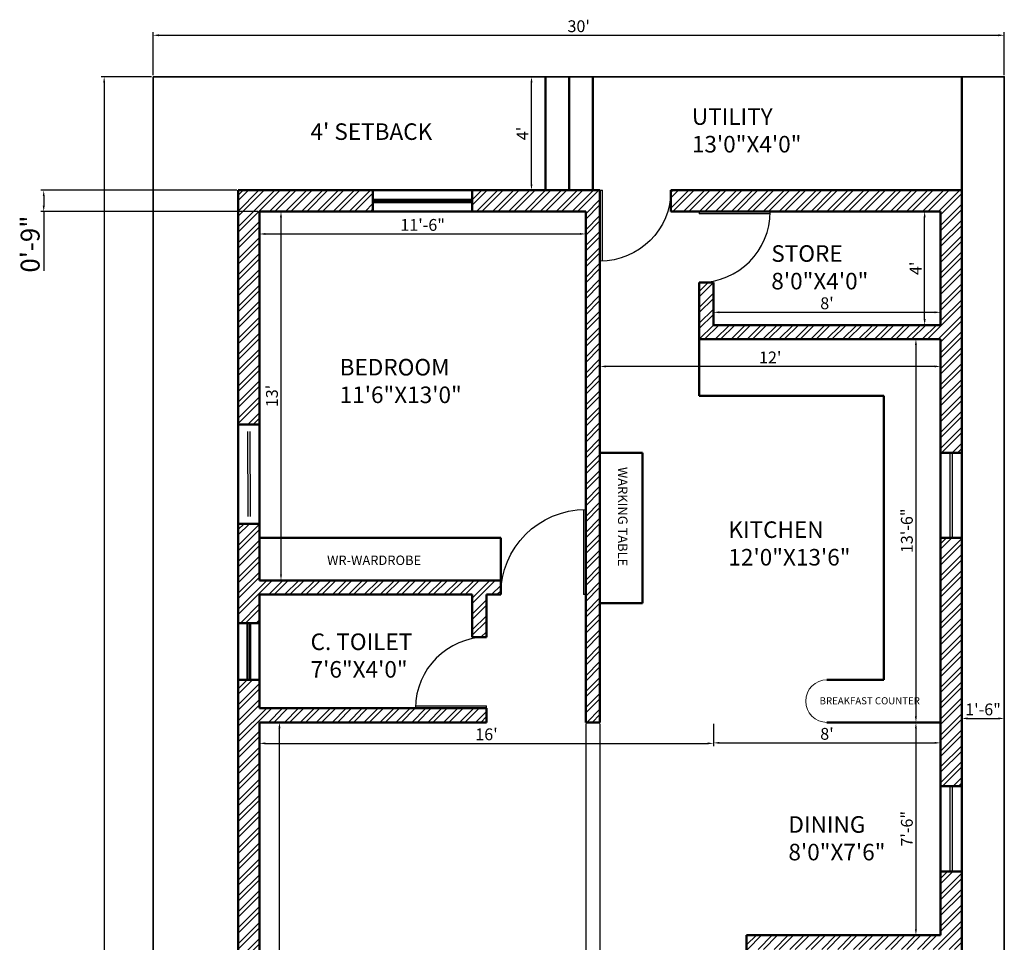
# Model space of a CAD drawing. Units: inches. Extents: x 1986 to 21484, y -1816 to 2016.
# Tile 83 of 85: x 4780 to 5197, y 1535 to 1925. Entities that reach past the tile are written whole.
import ezdxf

# ---------------------------------------------------------------- set-up
doc = ezdxf.new("R2010")
doc.units = ezdxf.units.IN
for name, color, linetype, lineweight in [('A-ANNO-DIMS', 2, 'Continuous', 18), ('A-ANNO-TEXT', 7, 'Continuous', 18), ('A-AREA-IDEN', 3, 'Continuous', 18), ('A-DOOR', 3, 'Continuous', 25), ('A-FURN', 8, 'Continuous', 18), ('A-GLAZ', 4, 'Continuous', 25), ('A-WALL', 7, 'Continuous', 50), ('A-WALL-PATT', 8, 'Continuous', 13), ('C-PROP', 7, 'Continuous', 35)]:
    doc.layers.add(name, color=color, linetype=linetype, lineweight=lineweight)
doc.styles.get("Standard").update_dxf_attribs({"font": 'arial.ttf'})
doc.dimstyles.new('ISO-25', dxfattribs={"dimtxt": 8, "dimasz": 2.5, "dimexe": 1.25, "dimexo": 0.625, "dimtad": 1, "dimdec": 1, "dimlunit": 3, "dimtxsty": 'Standard', "dimcen": 2.5, "dimadec": 0, "dimazin": 0, "dimtfac": 1, "dimtdec": 1, "dimtmove": 0, "dimatfit": 3, "dimfxl": 1, "dimarcsym": 0})

# ---------------------------------------------------------------- blocks, each defined once
blk = doc.blocks.new('D2')
for p, q in [((1722.5, 1505.46), (1722.5, 1475.46)), ((1723.5, 1505.46), (1723.5, 1475.46)), ((1722.5, 1475.46), (1723.5, 1475.46))]:
    blk.add_line(p, q)
blk.add_arc((1722.5, 1475.46), 30, 0, 90)
blk = doc.blocks.new('D1')
for p, q in [((1805.96, 1500.36), (1805.96, 1464.36)), ((1806.96, 1500.36), (1806.96, 1464.36)), ((1805.96, 1464.36), (1806.96, 1464.36))]:
    blk.add_line(p, q)
blk.add_arc((1805.96, 1464.36), 36, 0, 90)
blk = doc.blocks.new('*D35')
at = {"layer": 'A-ANNO-DIMS', "color": 0, "lineweight": -2, "transparency": 16777216}
for p, q in [((4882.51, 1843.75), (4892.24, 1843.75)), ((4890.99, 1690.25), (4890.99, 1841.25)), ((4882.51, 1687.75), (4892.24, 1687.75))]:
    blk.add_line(p, q, dxfattribs=at)
at = {"layer": 'A-ANNO-DIMS', "color": 0, "transparency": 16777216}
for points in [[(4890.57, 1841.25), (4891.4, 1841.25), (4890.99, 1843.75)], [(4890.57, 1690.25), (4891.4, 1690.25), (4890.99, 1687.75)]]:
    blk.add_solid(points, dxfattribs=at)
at = {"layer": 'Defpoints', "color": 0, "transparency": 16777216}
for p in [(4881.89, 1843.75), (4890.99, 1843.75), (4881.89, 1687.75)]:
    blk.add_point(p, dxfattribs=at)
at = {"layer": 'A-ANNO-DIMS', "color": 0, "transparency": 16777216, "insert": (4887.81, 1765.75), "char_height": 5, "attachment_point": 5, "rotation": 90}
blk.add_mtext("13'", dxfattribs=at)
blk = doc.blocks.new('*D36')
at = {"layer": 'A-ANNO-DIMS', "color": 0, "lineweight": -2, "transparency": 16777216}
for p, q in [((4881.89, 1843.13), (4881.89, 1833.02)), ((5019.89, 1843.13), (5019.89, 1833.02)), ((4884.39, 1834.27), (5017.39, 1834.27))]:
    blk.add_line(p, q, dxfattribs=at)
at = {"layer": 'A-ANNO-DIMS', "color": 0, "transparency": 16777216}
for points in [[(4884.39, 1834.68), (4884.39, 1833.85), (4881.89, 1834.27)], [(5017.39, 1834.68), (5017.39, 1833.85), (5019.89, 1834.27)]]:
    blk.add_solid(points, dxfattribs=at)
at = {"layer": 'Defpoints', "color": 0, "transparency": 16777216}
for p in [(4881.89, 1843.75), (5019.89, 1843.75), (5019.89, 1834.27)]:
    blk.add_point(p, dxfattribs=at)
at = {"layer": 'A-ANNO-DIMS', "color": 0, "transparency": 16777216, "insert": (4950.89, 1837.44), "char_height": 5, "attachment_point": 5}
blk.add_mtext('11\'-6"', dxfattribs=at)
blk = doc.blocks.new('*D37')
at = {"layer": 'A-ANNO-DIMS', "color": 0, "lineweight": -2, "transparency": 16777216}
for p, q in [((5169.26, 1843.75), (5161.95, 1843.75)), ((5163.2, 1798.25), (5163.2, 1841.25)), ((5169.26, 1795.75), (5161.95, 1795.75))]:
    blk.add_line(p, q, dxfattribs=at)
at = {"layer": 'A-ANNO-DIMS', "color": 0, "transparency": 16777216}
for points in [[(5162.78, 1841.25), (5163.62, 1841.25), (5163.2, 1843.75)], [(5162.78, 1798.25), (5163.62, 1798.25), (5163.2, 1795.75)]]:
    blk.add_solid(points, dxfattribs=at)
at = {"layer": 'Defpoints', "color": 0, "transparency": 16777216}
for p in [(5163.2, 1843.75), (5169.89, 1843.75), (5169.89, 1795.75)]:
    blk.add_point(p, dxfattribs=at)
at = {"layer": 'A-ANNO-DIMS', "color": 0, "transparency": 16777216, "insert": (5160.07, 1819.75), "char_height": 5, "attachment_point": 5, "rotation": 90}
blk.add_mtext("4'", dxfattribs=at)
blk = doc.blocks.new('*D38')
at = {"layer": 'A-ANNO-DIMS', "color": 0, "lineweight": -2, "transparency": 16777216}
for p, q in [((5073.89, 1796.38), (5073.89, 1802.38)), ((5076.39, 1801.13), (5167.39, 1801.13)), ((5169.89, 1796.38), (5169.89, 1802.38))]:
    blk.add_line(p, q, dxfattribs=at)
at = {"layer": 'A-ANNO-DIMS', "color": 0, "transparency": 16777216}
for points in [[(5076.39, 1801.54), (5076.39, 1800.71), (5073.89, 1801.13)], [(5167.39, 1801.54), (5167.39, 1800.71), (5169.89, 1801.13)]]:
    blk.add_solid(points, dxfattribs=at)
at = {"layer": 'Defpoints', "color": 0, "transparency": 16777216}
for p in [(5169.89, 1801.13), (5073.89, 1795.75), (5169.89, 1795.75)]:
    blk.add_point(p, dxfattribs=at)
at = {"layer": 'A-ANNO-DIMS', "color": 0, "transparency": 16777216, "insert": (5121.89, 1804.31), "char_height": 5, "attachment_point": 5}
blk.add_mtext("8'", dxfattribs=at)
blk = doc.blocks.new('*D39')
at = {"layer": 'A-ANNO-DIMS', "color": 0, "lineweight": -2, "transparency": 16777216}
for p, q in [((5025.89, 1789.13), (5025.89, 1777)), ((5169.89, 1789.13), (5169.89, 1777)), ((5167.39, 1778.25), (5028.39, 1778.25))]:
    blk.add_line(p, q, dxfattribs=at)
at = {"layer": 'A-ANNO-DIMS', "color": 0, "transparency": 16777216}
for points in [[(5028.39, 1778.67), (5028.39, 1777.84), (5025.89, 1778.25)], [(5167.39, 1778.67), (5167.39, 1777.84), (5169.89, 1778.25)]]:
    blk.add_solid(points, dxfattribs=at)
at = {"layer": 'Defpoints', "color": 0, "transparency": 16777216}
for p in [(5025.89, 1789.75), (5169.89, 1789.75), (5025.89, 1778.25)]:
    blk.add_point(p, dxfattribs=at)
at = {"layer": 'A-ANNO-DIMS', "color": 0, "transparency": 16777216, "insert": (5097.89, 1781.39), "char_height": 5, "attachment_point": 5}
blk.add_mtext("12'", dxfattribs=at)
blk = doc.blocks.new('*D40')
at = {"layer": 'A-ANNO-DIMS', "color": 0, "lineweight": -2, "transparency": 16777216}
for p, q in [((5169.26, 1789.75), (5158.26, 1789.75)), ((5159.51, 1787.25), (5159.51, 1630.25)), ((5169.26, 1627.75), (5158.26, 1627.75))]:
    blk.add_line(p, q, dxfattribs=at)
at = {"layer": 'A-ANNO-DIMS', "color": 0, "transparency": 16777216}
for points in [[(5159.09, 1787.25), (5159.92, 1787.25), (5159.51, 1789.75)], [(5159.09, 1630.25), (5159.92, 1630.25), (5159.51, 1627.75)]]:
    blk.add_solid(points, dxfattribs=at)
at = {"layer": 'Defpoints', "color": 0, "transparency": 16777216}
for p in [(5169.89, 1789.75), (5159.51, 1627.75), (5169.89, 1627.75)]:
    blk.add_point(p, dxfattribs=at)
at = {"layer": 'A-ANNO-DIMS', "color": 0, "transparency": 16777216, "insert": (5156.33, 1708.75), "char_height": 5, "attachment_point": 5, "rotation": 90}
blk.add_mtext('13\'-6"', dxfattribs=at)
blk = doc.blocks.new('*D41')
at = {"layer": 'A-ANNO-DIMS', "color": 0, "lineweight": -2, "transparency": 16777216}
for p, q in [((5169.26, 1627.75), (5158.26, 1627.75)), ((5159.51, 1625.25), (5159.51, 1540.25)), ((5169.26, 1537.75), (5158.26, 1537.75))]:
    blk.add_line(p, q, dxfattribs=at)
at = {"layer": 'A-ANNO-DIMS', "color": 0, "transparency": 16777216}
for points in [[(5159.09, 1625.25), (5159.92, 1625.25), (5159.51, 1627.75)], [(5159.09, 1540.25), (5159.92, 1540.25), (5159.51, 1537.75)]]:
    blk.add_solid(points, dxfattribs=at)
at = {"layer": 'Defpoints', "color": 0, "transparency": 16777216}
for p in [(5169.89, 1627.75), (5159.51, 1537.75), (5169.89, 1537.75)]:
    blk.add_point(p, dxfattribs=at)
at = {"layer": 'A-ANNO-DIMS', "color": 0, "transparency": 16777216, "insert": (5156.33, 1582.75), "char_height": 5, "attachment_point": 5, "rotation": 90}
blk.add_mtext('7\'-6"', dxfattribs=at)
blk = doc.blocks.new('*D42')
at = {"layer": 'A-ANNO-DIMS', "color": 0, "lineweight": -2, "transparency": 16777216}
for p, q in [((4882.51, 1627.75), (4891.58, 1627.75)), ((4890.33, 1390.25), (4890.33, 1625.25)), ((4882.51, 1387.75), (4891.58, 1387.75))]:
    blk.add_line(p, q, dxfattribs=at)
at = {"layer": 'A-ANNO-DIMS', "color": 0, "transparency": 16777216}
for points in [[(4889.91, 1625.25), (4890.74, 1625.25), (4890.33, 1627.75)], [(4889.91, 1390.25), (4890.74, 1390.25), (4890.33, 1387.75)]]:
    blk.add_solid(points, dxfattribs=at)
at = {"layer": 'Defpoints', "color": 0, "transparency": 16777216}
for p in [(4881.89, 1627.75), (4890.33, 1627.75), (4881.89, 1387.75)]:
    blk.add_point(p, dxfattribs=at)
at = {"layer": 'A-ANNO-DIMS', "color": 0, "transparency": 16777216, "insert": (4887.15, 1507.75), "char_height": 5, "attachment_point": 5, "rotation": 90}
blk.add_mtext("20'", dxfattribs=at)
blk = doc.blocks.new('*D43')
at = {"layer": 'A-ANNO-DIMS', "color": 0, "lineweight": -2, "transparency": 16777216}
for p, q in [((4881.89, 1627.13), (4881.89, 1617.62)), ((5073.89, 1627.13), (5073.89, 1617.62)), ((4884.39, 1618.87), (5071.39, 1618.87))]:
    blk.add_line(p, q, dxfattribs=at)
at = {"layer": 'A-ANNO-DIMS', "color": 0, "transparency": 16777216}
for points in [[(4884.39, 1619.28), (4884.39, 1618.45), (4881.89, 1618.87)], [(5071.39, 1619.28), (5071.39, 1618.45), (5073.89, 1618.87)]]:
    blk.add_solid(points, dxfattribs=at)
at = {"layer": 'Defpoints', "color": 0, "transparency": 16777216}
for p in [(4881.89, 1627.75), (5073.89, 1627.75), (5073.89, 1618.87)]:
    blk.add_point(p, dxfattribs=at)
at = {"layer": 'A-ANNO-DIMS', "color": 0, "transparency": 16777216, "insert": (4977.89, 1622.05), "char_height": 5, "attachment_point": 5}
blk.add_mtext("16'", dxfattribs=at)
blk = doc.blocks.new('*D44')
at = {"layer": 'A-ANNO-DIMS', "color": 0, "lineweight": -2, "transparency": 16777216}
for p, q in [((5073.89, 1627.13), (5073.89, 1617.83)), ((5169.89, 1612.9), (5169.89, 1620.33)), ((5076.39, 1619.08), (5167.39, 1619.08))]:
    blk.add_line(p, q, dxfattribs=at)
at = {"layer": 'A-ANNO-DIMS', "color": 0, "transparency": 16777216}
for points in [[(5076.39, 1619.49), (5076.39, 1618.66), (5073.89, 1619.08)], [(5167.39, 1619.49), (5167.39, 1618.66), (5169.89, 1619.08)]]:
    blk.add_solid(points, dxfattribs=at)
at = {"layer": 'Defpoints', "color": 0, "transparency": 16777216}
for p in [(5073.89, 1627.75), (5169.89, 1619.08), (5169.89, 1612.28)]:
    blk.add_point(p, dxfattribs=at)
at = {"layer": 'A-ANNO-DIMS', "color": 0, "transparency": 16777216, "insert": (5121.89, 1622.25), "char_height": 5, "attachment_point": 5}
blk.add_mtext("8'", dxfattribs=at)
blk = doc.blocks.new('*D78')
at = {"layer": 'A-ANNO-DIMS', "color": 0, "lineweight": -2, "transparency": 16777216}
for p, q in [((4997.55, 1900.75), (4998.17, 1900.75)), ((4996.92, 1855.25), (4996.92, 1898.25)), ((4997.55, 1852.75), (4998.17, 1852.75))]:
    blk.add_line(p, q, dxfattribs=at)
at = {"layer": 'A-ANNO-DIMS', "color": 0, "transparency": 16777216}
for points in [[(4996.51, 1898.25), (4997.34, 1898.25), (4996.92, 1900.75)], [(4996.51, 1855.25), (4997.34, 1855.25), (4996.92, 1852.75)]]:
    blk.add_solid(points, dxfattribs=at)
at = {"layer": 'Defpoints', "color": 0, "transparency": 16777216}
for p in [(4996.92, 1900.75), (4996.92, 1900.75), (4996.92, 1852.75)]:
    blk.add_point(p, dxfattribs=at)
at = {"layer": 'A-ANNO-DIMS', "color": 0, "transparency": 16777216, "insert": (4993.8, 1876.75), "char_height": 5, "attachment_point": 5, "rotation": 90}
blk.add_mtext("4'", dxfattribs=at)
blk = doc.blocks.new('*D79')
at = {"layer": 'A-ANNO-DIMS', "color": 0, "lineweight": -2, "transparency": 16777216}
for p, q in [((5178.89, 1630.03), (5178.89, 1630.65)), ((5181.39, 1629.4), (5194.39, 1629.4)), ((5196.89, 1630.03), (5196.89, 1630.65))]:
    blk.add_line(p, q, dxfattribs=at)
at = {"layer": 'A-ANNO-DIMS', "color": 0, "transparency": 16777216}
for points in [[(5181.39, 1629.82), (5181.39, 1628.98), (5178.89, 1629.4)], [(5194.39, 1629.82), (5194.39, 1628.98), (5196.89, 1629.4)]]:
    blk.add_solid(points, dxfattribs=at)
at = {"layer": 'Defpoints', "color": 0, "transparency": 16777216}
for p in [(5178.89, 1629.4), (5196.89, 1629.4), (5196.89, 1629.4)]:
    blk.add_point(p, dxfattribs=at)
at = {"layer": 'A-ANNO-DIMS', "color": 0, "transparency": 16777216, "insert": (5187.89, 1632.58), "char_height": 5, "attachment_point": 5}
blk.add_mtext('1\'-6"', dxfattribs=at)
blk = doc.blocks.new('*D81')
at = {"layer": 'A-ANNO-DIMS', "color": 0, "lineweight": -2, "transparency": 16777216}
for p, q in [((4836.26, 1900.75), (4814.95, 1900.75)), ((4816.2, 1898.25), (4816.2, 1069.25)), ((4836.26, 1066.75), (4814.95, 1066.75))]:
    blk.add_line(p, q, dxfattribs=at)
at = {"layer": 'A-ANNO-DIMS', "color": 0, "transparency": 16777216}
for points in [[(4815.78, 1898.25), (4816.61, 1898.25), (4816.2, 1900.75)], [(4815.78, 1069.25), (4816.61, 1069.25), (4816.2, 1066.75)]]:
    blk.add_solid(points, dxfattribs=at)
at = {"layer": 'Defpoints', "color": 0, "transparency": 16777216}
for p in [(4836.89, 1900.75), (4816.2, 1066.75), (4836.89, 1066.75)]:
    blk.add_point(p, dxfattribs=at)
at = {"layer": 'A-ANNO-DIMS', "color": 0, "transparency": 16777216, "insert": (4813.02, 1483.75), "char_height": 5, "attachment_point": 5, "rotation": 90}
blk.add_mtext('69\'-6"', dxfattribs=at)
blk = doc.blocks.new('*D82')
at = {"layer": 'A-ANNO-DIMS', "color": 0, "lineweight": -2, "transparency": 16777216}
for p, q in [((4836.89, 1901.38), (4836.89, 1919.52)), ((4839.39, 1918.27), (5194.39, 1918.27)), ((5196.89, 1901.38), (5196.89, 1919.52))]:
    blk.add_line(p, q, dxfattribs=at)
at = {"layer": 'A-ANNO-DIMS', "color": 0, "transparency": 16777216}
for points in [[(4839.39, 1918.69), (4839.39, 1917.86), (4836.89, 1918.27)], [(5194.39, 1918.69), (5194.39, 1917.86), (5196.89, 1918.27)]]:
    blk.add_solid(points, dxfattribs=at)
at = {"layer": 'Defpoints', "color": 0, "transparency": 16777216}
for p in [(5196.89, 1918.27), (4836.89, 1900.75), (5196.89, 1900.75)]:
    blk.add_point(p, dxfattribs=at)
at = {"layer": 'A-ANNO-DIMS', "color": 0, "transparency": 16777216, "insert": (5016.89, 1921.45), "char_height": 5, "attachment_point": 5}
blk.add_mtext("30'", dxfattribs=at)
blk = doc.blocks.new('WIN-36')
for p, q in [((0, 36), (0, 0)), ((0, 36), (0, 0)), ((1, 36), (1, 0))]:
    blk.add_line(p, q)
blk = doc.blocks.new('*D131')
at = {"layer": 'A-ANNO-DIMS', "color": 0, "lineweight": -2, "transparency": 16777216}
for p, q in [((4872.26, 1852.75), (4789.39, 1852.75)), ((4790.64, 1850.25), (4790.64, 1846.25)), ((4881.26, 1843.75), (4789.39, 1843.75)), ((4790.64, 1843.75), (4790.64, 1818.74))]:
    blk.add_line(p, q, dxfattribs=at)
at = {"layer": 'A-ANNO-DIMS', "color": 0, "transparency": 16777216}
for points in [[(4790.22, 1850.25), (4791.06, 1850.25), (4790.64, 1852.75)], [(4790.22, 1846.25), (4791.06, 1846.25), (4790.64, 1843.75)]]:
    blk.add_solid(points, dxfattribs=at)
at = {"layer": 'Defpoints', "color": 0, "transparency": 16777216}
for p in [(4872.89, 1852.75), (4790.64, 1843.75), (4881.89, 1843.75)]:
    blk.add_point(p, dxfattribs=at)
at = {"layer": 'A-ANNO-DIMS', "color": 0, "transparency": 16777216, "insert": (4785.93, 1829.99), "char_height": 8, "attachment_point": 5, "rotation": 90}
blk.add_mtext('0\'-9"', dxfattribs=at)
blk = doc.blocks.new('*D132')
at = {"layer": 'A-ANNO-DIMS', "color": 0, "lineweight": -2, "transparency": 16777216}
for p, q in [((5019.89, 1627.13), (5019.89, 953.11)), ((5025.89, 1627.13), (5025.89, 953.11)), ((5017.39, 954.36), (5014.89, 954.36)), ((5019.89, 954.36), (5025.89, 954.36)), ((5028.39, 954.36), (5053.4, 954.36))]:
    blk.add_line(p, q, dxfattribs=at)
at = {"layer": 'A-ANNO-DIMS', "color": 0, "transparency": 16777216}
for points in [[(5017.39, 954.78), (5017.39, 953.95), (5019.89, 954.36)], [(5028.39, 954.78), (5028.39, 953.95), (5025.89, 954.36)]]:
    blk.add_solid(points, dxfattribs=at)
at = {"layer": 'Defpoints', "color": 0, "transparency": 16777216}
for p in [(5019.89, 1627.75), (5025.89, 1627.75), (5025.89, 954.36)]:
    blk.add_point(p, dxfattribs=at)
at = {"layer": 'A-ANNO-DIMS', "color": 0, "transparency": 16777216, "insert": (5042.15, 959.07), "char_height": 8, "attachment_point": 5}
blk.add_mtext('0\'-6"', dxfattribs=at)

msp = doc.modelspace()

# ---------------------------------------------------------------- hatches: boundary and pattern name
at = {"layer": 'A-WALL-PATT'}
h = msp.add_hatch(dxfattribs=at)
h.set_pattern_fill('ANSI32', color=256, scale=0.5)
h.set_pattern_definition([(45, (1297.9813, 0), (-3.367596, 3.367596), []), (45, (1300.2263, 0), (-3.367596, 3.367596), [])])
h.paths.add_polyline_path([(4929.89, 1852.75), (4872.89, 1852.75), (4872.89, 1753.75), (4881.89, 1753.75), (4881.89, 1843.75), (4929.89, 1843.75)])
h.paths.add_polyline_path([(5025.89, 1852.75), (4971.89, 1852.75), (4971.89, 1843.75), (5019.89, 1843.75), (5019.89, 1627.75), (5025.89, 1627.75)])
h.paths.add_polyline_path([(5178.89, 1852.75), (5055.89, 1852.75), (5055.89, 1843.75), (5169.89, 1843.75), (5169.89, 1795.75), (5073.89, 1795.75), (5073.89, 1813.75), (5067.89, 1813.75), (5067.89, 1789.75), (5169.89, 1789.75), (5169.89, 1741.75), (5178.89, 1741.75)])
h.paths.add_polyline_path([(5178.89, 1705.75), (5169.89, 1705.75), (5169.89, 1600.75), (5178.89, 1600.75)])
h.paths.add_polyline_path([(4983.89, 1687.75), (4881.89, 1687.75), (4881.89, 1711.75), (4872.89, 1711.75), (4872.89, 1669.75), (4881.89, 1669.75), (4881.89, 1681.75), (4971.89, 1681.75), (4971.89, 1663.75), (4977.89, 1663.75), (4977.89, 1681.75), (4983.89, 1681.75)])
h.paths.add_polyline_path([(4881.89, 1399.75), (4872.89, 1399.75), (4872.89, 1276.75), (4881.89, 1276.75)])
h.paths.add_polyline_path([(4946.39, 1387.75), (4929.89, 1387.75), (4929.89, 1378.75), (4946.39, 1378.75)])
h.paths.add_polyline_path([(5013.89, 1387.75), (4988.39, 1387.75), (4988.39, 1378.75), (5004.89, 1378.75), (5004.89, 1189.75), (5013.89, 1189.75)])
h.paths.add_polyline_path([(5178.89, 1387.75), (5169.89, 1387.75), (5049.89, 1387.75), (5049.89, 1381.75), (5169.89, 1381.75), (5169.89, 1363.75), (5178.89, 1363.75)])
h.paths.add_polyline_path([(5178.89, 1441.75), (5169.89, 1441.75), (5169.89, 1423.75), (5178.89, 1423.75)])
h.paths.add_polyline_path([(5178.89, 1495.75), (5169.89, 1495.75), (5169.89, 1477.75), (5178.89, 1477.75)])
h.paths.add_polyline_path([(5178.89, 1339.75), (5169.89, 1339.75), (5169.89, 1321.75), (5073.89, 1321.75), (5073.89, 1351.75), (5067.89, 1351.75), (5067.89, 1315.75), (5169.89, 1315.75), (5169.89, 1303.75), (5178.89, 1303.75)])
h.paths.add_polyline_path([(5178.89, 1261.75), (5169.89, 1261.75), (5169.89, 1189.75), (5178.89, 1189.75)])
h.paths.add_polyline_path([(5178.89, 1147.75), (5169.89, 1147.75), (5169.89, 1123.75), (5061.89, 1123.75), (5061.89, 1114.75), (5178.89, 1114.75)])
h.paths.add_polyline_path([(5019.89, 1123.75), (5013.89, 1123.75), (5013.89, 1147.75), (5004.89, 1147.75), (5004.89, 1114.75), (5019.89, 1114.75)])
h.paths.add_polyline_path([(5178.89, 1564.75), (5169.89, 1564.75), (5169.89, 1537.75), (5087.89, 1537.75), (5087.89, 1531.75), (5169.89, 1531.75), (5178.89, 1531.75)])
h.paths.add_polyline_path([(4881.89, 1627.75), (4977.89, 1627.75), (4977.89, 1633.75), (4947.89, 1633.75), (4881.89, 1633.75), (4881.89, 1645.75), (4872.89, 1645.75), (4872.89, 1441.75), (4881.89, 1441.75)])
h.paths.add_polyline_path([(5031.24, 1736.83), (5031.24, 1685.78), (5039.78, 1685.78), (5039.78, 1736.83)], flags=9)
h.paths.add_polyline_path([(5061.79, 1864.73), (5110.75, 1864.73), (5110.75, 1891.35), (5061.79, 1891.35)], flags=9)
h.paths.add_polyline_path([(5095.95, 1806.84), (5139.77, 1806.84), (5139.77, 1833.45), (5095.95, 1833.45)], flags=25)
h.paths.add_polyline_path([(5077.23, 1690.08), (5131.36, 1690.08), (5131.36, 1716.69), (5077.23, 1716.69)], flags=9)
h.paths.add_polyline_path([(5103.21, 1565.41), (5147.01, 1565.41), (5147.01, 1592.03), (5103.21, 1592.03)], flags=9)
h.paths.add_polyline_path([(4936.55, 1496.24), (5009.24, 1496.24), (5009.24, 1522.85), (4936.55, 1522.85)], flags=9)
h.paths.add_polyline_path([(4915.95, 1320.51), (4964.91, 1320.51), (4964.91, 1347.12), (4915.95, 1347.12)], flags=9)
h.paths.add_polyline_path([(5066.5, 1208.98), (5134.5, 1208.98), (5134.5, 1235.59), (5066.5, 1235.59)], flags=9)
h.paths.add_polyline_path([(5089.68, 1338.54), (5142.51, 1338.54), (5142.51, 1365.15), (5089.68, 1365.15)], flags=9)
h.paths.add_polyline_path([(4912.83, 1758.76), (4969.06, 1758.76), (4969.06, 1785.38), (4912.83, 1785.38)], flags=9)
h.paths.add_polyline_path([(4901.36, 1642.68), (4953.09, 1642.68), (4953.09, 1669.29), (4901.36, 1669.29)], flags=9)

# ---------------------------------------------------------------- linework, layer by layer
at = {"layer": 'A-FURN'}
msp.add_arc((5121.89, 1636.75), 9, 90, 270, dxfattribs=at)
at = {"layer": 'A-WALL'}
for p, q in [((5002.89, 1900.75), (5002.89, 1852.75)), ((5012.89, 1900.75), (5012.89, 1852.75)), ((5022.89, 1900.75), (5022.89, 1852.75)), ((5178.89, 1900.75), (5178.89, 1114.75)), ((4872.89, 1852.75), (5025.89, 1852.75)), ((4872.89, 1276.75), (4872.89, 1852.75)), ((4929.89, 1843.75), (4929.89, 1852.75)), ((4971.89, 1843.75), (4971.89, 1852.75)), ((5025.89, 1627.75), (5025.89, 1852.75)), ((5055.89, 1852.75), (5178.89, 1852.75)), ((5055.89, 1843.75), (5055.89, 1852.75)), ((4929.89, 1848.75), (4971.89, 1848.75)), ((4929.89, 1847.75), (4971.89, 1847.75)), ((4881.89, 1843.75), (5019.89, 1843.75)), ((4881.89, 1687.75), (4881.89, 1843.75)), ((5019.89, 1627.75), (5019.89, 1843.75)), ((5055.89, 1843.75), (5169.89, 1843.75)), ((5169.89, 1843.75), (5169.89, 1795.75)), ((5067.89, 1813.75), (5073.89, 1813.75)), ((5067.89, 1813.75), (5067.89, 1765.75)), ((5073.89, 1813.75), (5073.89, 1795.75)), ((5073.89, 1795.75), (5169.89, 1795.75)), ((5067.89, 1789.75), (5169.89, 1789.75)), ((5169.89, 1789.75), (5169.89, 1537.75)), ((5067.89, 1765.75), (5145.89, 1765.75)), ((5145.89, 1765.75), (5145.89, 1645.75)), ((4872.89, 1753.75), (4881.89, 1753.75)), ((5025.89, 1741.75), (5043.89, 1741.75)), ((5043.89, 1678.13), (5043.89, 1741.75)), ((5169.89, 1741.75), (5178.89, 1741.75)), ((4872.89, 1711.75), (4881.89, 1711.75)), ((4881.89, 1705.75), (4983.89, 1705.75)), ((4983.89, 1681.75), (4983.89, 1705.75)), ((5169.89, 1705.75), (5178.89, 1705.75)), ((4881.89, 1687.75), (4983.89, 1687.75)), ((4881.89, 1681.75), (4971.89, 1681.75)), ((4881.89, 1633.75), (4881.89, 1681.75)), ((4971.89, 1663.75), (4971.89, 1681.75)), ((4977.89, 1681.75), (4983.89, 1681.75)), ((4977.89, 1663.75), (4977.89, 1681.75)), ((5025.89, 1678.13), (5043.89, 1678.13)), ((4872.89, 1669.75), (4881.89, 1669.75)), ((4876.89, 1645.75), (4876.89, 1669.75)), ((4877.89, 1645.75), (4877.89, 1669.75)), ((4971.89, 1663.75), (4977.89, 1663.75)), ((4872.89, 1645.75), (4881.89, 1645.75)), ((5121.89, 1645.75), (5145.89, 1645.75)), ((4881.89, 1633.75), (4977.89, 1633.75)), ((4977.89, 1627.75), (4977.89, 1633.75)), ((4881.89, 1276.75), (4881.89, 1627.75)), ((4881.89, 1627.75), (4977.89, 1627.75)), ((5019.89, 1627.75), (5025.89, 1627.75)), ((5121.89, 1627.75), (5169.89, 1627.75)), ((5169.89, 1600.75), (5178.89, 1600.75)), ((5169.89, 1564.75), (5178.89, 1564.75)), ((5087.89, 1537.75), (5087.89, 1489.75)), ((5087.89, 1537.75), (5169.89, 1537.75))]:
    msp.add_line(p, q, dxfattribs=at)
at = {"layer": 'C-PROP'}
msp.add_lwpolyline([(4836.89, 1900.75), (5196.89, 1900.75), (5196.89, 1066.75), (4836.89, 1066.75)], close=True, dxfattribs=at)

# ---------------------------------------------------------------- block references
at = {"layer": 'A-DOOR', "xscale": -1, "rotation": 180}
msp.add_blockref('D2', (3303.39, 3328.21), dxfattribs=at)
at = {"layer": 'A-DOOR'}
for p, rotation in [((3592.43, 3566.25), 270), ((6453.35, -88.75), 90)]:
    msp.add_blockref('D2', p, dxfattribs=dict(at, rotation=rotation))
at = {"layer": 'A-DOOR', "xscale": -1}
msp.add_blockref('D1', (6825.85, 217.39), dxfattribs=at)
at = {"layer": 'A-GLAZ', "rotation": 0.3027934322012576}
msp.add_blockref('WIN-36', (4876.98, 1714.75), dxfattribs=at)
at = {"layer": 'A-GLAZ'}
for p in [(5173.89, 1705.75), (5173.89, 1564.75)]:
    msp.add_blockref('WIN-36', p, dxfattribs=at)

# ---------------------------------------------------------------- texts
at = {"layer": 'A-ANNO-TEXT', "attachment_point": 1}
for s, insert, char_height in [("{\\fTimes New Roman|b0|i0|c0|p18;4' SETBACK}", (4903.46, 1881.03), 7), ('{\\fTimes New Roman|b0|i0|c0|p18;WR-WARDROBE}', (4910.47, 1698.29), 4), ('{\\fTimes New Roman|b0|i0|c0|p18;BREAKFAST COUNTER}', (5118.78, 1638.37), 3)]:
    msp.add_mtext_dynamic_manual_height_columns(s, width=105.6127, gutter_width=12.5, heights=[0], dxfattribs=dict(at, insert=insert, char_height=char_height))
at = {"layer": 'A-ANNO-TEXT', "insert": (5037.52, 1735.75), "char_height": 4, "attachment_point": 1, "rotation": 270}
msp.add_mtext_dynamic_manual_height_columns('{\\fTimes New Roman|b0|i0|c0|p18;WARKING TABLE}', width=105.6127, gutter_width=12.5, heights=[0], dxfattribs=at)
at = {"layer": 'A-AREA-IDEN', "char_height": 7, "attachment_point": 1}
for s, insert in [('{\\fTimes New Roman|b0|i0|c0|p18;UTILITY\\P13\'0"X4\'0"}', (5064.75, 1887.39)), ('{\\fTimes New Roman|b0|i0|c0|p18;STORE\\P8\'0"X4\'0"}', (5098.35, 1829.49)), ('{\\fTimes New Roman|b0|i0|c0|p18;BEDROOM \\P11\'6"X13\'0"}', (4915.79, 1781.42)), ('{\\fTimes New Roman|b0|i0|c0|p18;KITCHEN\\P12\'0"X13\'6"}', (5080.19, 1712.73)), ('{\\fTimes New Roman|b0|i0|c0|p18;C. TOILET\\P7\'6"X4\'0"}', (4903.49, 1665.33)), ('{\\fTimes New Roman|b0|i0|c0|p18;DINING\\P8\'0"X7\'6"}', (5105.58, 1588.07))]:
    msp.add_mtext_dynamic_manual_height_columns(s, width=105.6127, gutter_width=12.5, heights=[0], dxfattribs=dict(at, insert=insert))

# ---------------------------------------------------------------- dimensions: what is measured, and where the dimension line sits
at = {"layer": 'A-ANNO-DIMS'}
for base, p1, p2, override, picture, middle in [((5196.89, 1918.27), (4836.89, 1900.75), (5196.89, 1900.75), {"dimtxt": 5, "dimclrd": 0, "dimclre": 0, "dimclrt": 0}, '*D82', (5016.89, 1921.45)), ((5019.89, 1834.27), (4881.89, 1843.75), (5019.89, 1843.75), {"dimtxt": 5, "dimclrd": 0, "dimclre": 0, "dimclrt": 0}, '*D36', (4950.89, 1837.44)), ((5169.89, 1801.13), (5073.89, 1795.75), (5169.89, 1795.75), {"dimtxt": 5, "dimclrd": 0, "dimclre": 0, "dimclrt": 0}, '*D38', (5121.89, 1804.31)), ((5025.89, 1778.25), (5169.89, 1789.75), (5025.89, 1789.75), {"dimtxt": 5, "dimclrd": 0, "dimclre": 0, "dimclrt": 0}, '*D39', (5097.89, 1781.39)), ((5196.89, 1629.4), (5178.89, 1629.4), (5196.89, 1629.4), {"dimtxt": 5, "dimclrd": 0, "dimclre": 0, "dimclrt": 0}, '*D79', (5187.89, 1632.58)), ((5073.89, 1618.87), (4881.89, 1627.75), (5073.89, 1627.75), {"dimtxt": 5, "dimclrd": 0, "dimclre": 0, "dimclrt": 0}, '*D43', (4977.89, 1622.05)), ((5025.89, 954.36), (5019.89, 1627.75), (5025.89, 1627.75), {"dimdec": 1, "dimlfac": 1, "dimrnd": 0, "dimzin": 1, "dimdsep": 46, "dimlunit": 4, "dimfrac": 2}, '*D132', (5042.15, 959.07)), ((5169.89, 1619.08), (5073.89, 1627.75), (5169.89, 1612.28), {"dimtxt": 5, "dimclrd": 0, "dimclre": 0, "dimclrt": 0, "dimtmove": 1}, '*D44', (5121.89, 1622.25))]:
    dim = msp.add_linear_dim(base=base, p1=p1, p2=p2, dimstyle='ISO-25', override=override, dxfattribs=at)
    dim.commit()
    dim.dimension.update_dxf_attribs({"geometry": picture, "text_midpoint": middle})
for base, p1, p2, angle, override, picture, middle in [((4816.2, 1066.75), (4836.89, 1900.75), (4836.89, 1066.75), 90, {"dimtxt": 5, "dimclrd": 0, "dimclre": 0, "dimclrt": 0}, '*D81', (4813.02, 1483.75)), ((4996.92, 1900.75), (4996.92, 1852.75), (4996.92, 1900.75), 90, {"dimtxt": 5, "dimclrd": 0, "dimclre": 0, "dimclrt": 0}, '*D78', (4993.8, 1876.75)), ((4790.64, 1843.75), (4872.89, 1852.75), (4881.89, 1843.75), 90, {"dimdec": 1, "dimlfac": 1, "dimrnd": 0, "dimzin": 1, "dimdsep": 46, "dimlunit": 4, "dimfrac": 2}, '*D131', (4785.93, 1829.99)), ((4890.99, 1843.75), (4881.89, 1687.75), (4881.89, 1843.75), 270, {"dimtxt": 5, "dimclrd": 0, "dimclre": 0, "dimclrt": 0}, '*D35', (4887.81, 1765.75)), ((5163.2, 1843.75), (5169.89, 1795.75), (5169.89, 1843.75), 270, {"dimtxt": 5, "dimclrd": 0, "dimclre": 0, "dimclrt": 0}, '*D37', (5160.07, 1819.75)), ((5159.51, 1627.75), (5169.89, 1789.75), (5169.89, 1627.75), 90, {"dimtxt": 5, "dimclrd": 0, "dimclre": 0, "dimclrt": 0}, '*D40', (5156.33, 1708.75)), ((4890.33, 1627.75), (4881.89, 1387.75), (4881.89, 1627.75), 90, {"dimtxt": 5, "dimclrd": 0, "dimclre": 0, "dimclrt": 0}, '*D42', (4887.15, 1507.75)), ((5159.51, 1537.75), (5169.89, 1627.75), (5169.89, 1537.75), 90, {"dimtxt": 5, "dimclrd": 0, "dimclre": 0, "dimclrt": 0}, '*D41', (5156.33, 1582.75))]:
    dim = msp.add_linear_dim(base=base, p1=p1, p2=p2, angle=angle, dimstyle='ISO-25', override=override, dxfattribs=at)
    dim.commit()
    dim.dimension.update_dxf_attribs({"geometry": picture, "text_midpoint": middle})

doc.saveas('drawing.dxf')
